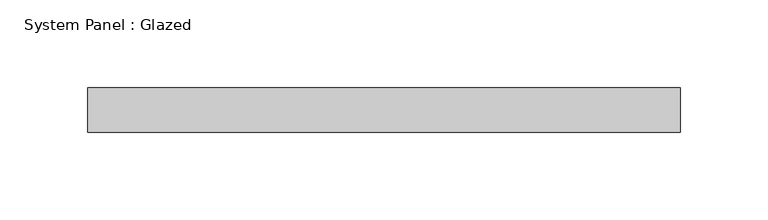
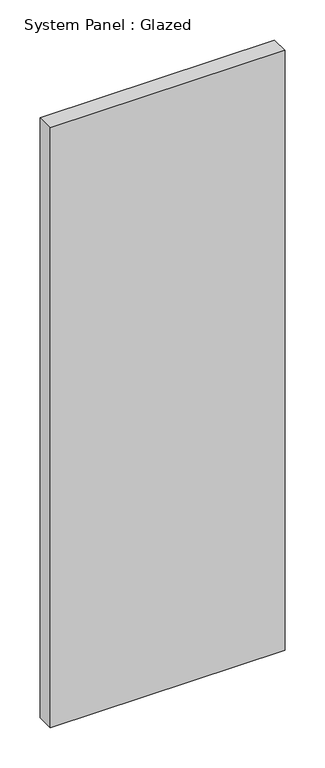
"""IFC4 building model written with IfcOpenShell, lengths in millimetres: plate geometry, System Panel : Glazed."""

from ifc_helpers import new_model, si_unit, origin, origin_with_axes, place, context, project, spatial, polyline, outline, extrude, source, transform, mapped, element, save


def system_panel_glazed_70ef586e(model_context):
    return source(origin(), model_context, "Body", "SweptSolid", [
        extrude(outline(polyline([(169.2946208, 19.05), (-169.2946208, 19.05), (-169.2946208, 44.45), (169.2946208, 44.45), (169.2946208, 19.05)])), origin_with_axes(), (0.0, 0.0, 1.0), 914.4),
    ])


if __name__ == "__main__":
    model = new_model("IFC4")
    model_context = context("Model", 3, world=origin())
    ifc_project = project(units=[si_unit("LENGTHUNIT", "METRE", prefix="MILLI")], contexts=[model_context])
    site = spatial("IfcSite", under=ifc_project)
    building = spatial("IfcBuilding", under=site)
    placement = place(None, origin())
    system_panel_glazed_shape = system_panel_glazed_70ef586e(model_context)
    element("IfcPlate", 1, ObjectType="System Panel : Glazed", at=placement, inside=building, context=model_context, shape_type="MappedRepresentation", body=[
        mapped(system_panel_glazed_shape, transform((0.0, 0.0, 0.0), x_axis=(1.0, 0.0, 0.0), y_axis=(0.0, 1.0, 0.0), z_axis=(0.0, 0.0, 1.0))),
    ])
    save(model, "model.ifc")

# Revit data of these elements
# Type "System Panel : Glazed"
#   Construction Type Id = "GSP4R"
#   Analytic Construction = "1/8 in Pilkington single glazing"
#   Visual Light Transmittance = 0.9
#   Solar Heat Gain Coefficient = 0.86
#   Heat Transfer Coefficient (U) = 1.18115 BTU/(h·ft²·°F)
# Element 1 (IfcPlate, "System Panel : Glazed")
#   Materials on its faces: "Glass"
# Materials
#   "Glass": class "Glass", colour RGB 0 128 192, transparency 0.75, Description = "Soda Lime Glass", Cost = 0
